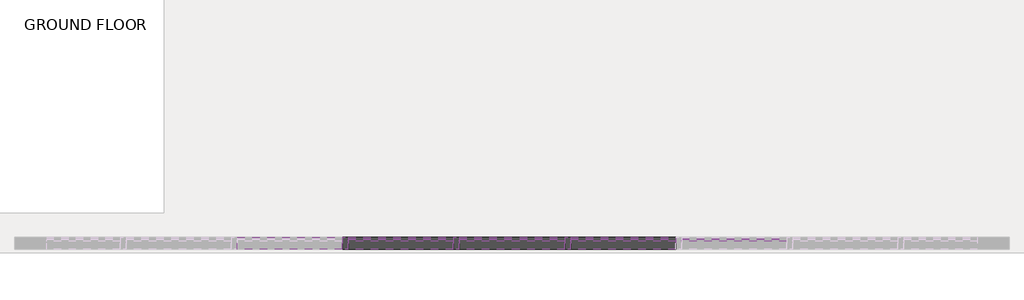
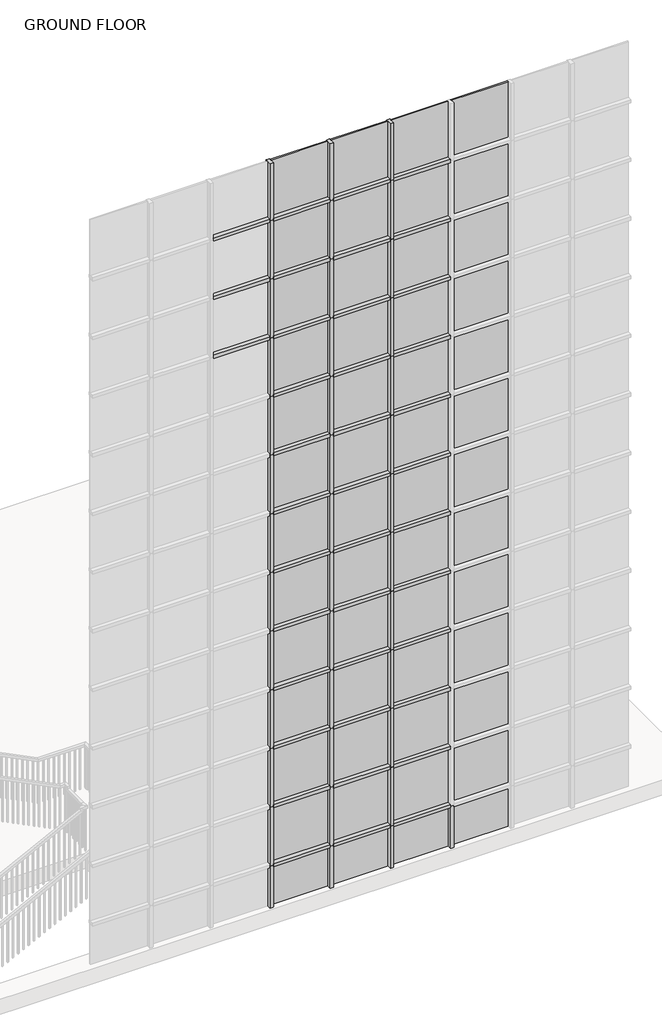
# One storey, part 4 of 16: 79 members, 52 plates.
"""IFC4 building model written with IfcOpenShell, lengths in millimetres."""

from ifc_helpers import new_model, si_unit, origin, place, context, project, spatial, transform, mapped, element, save
from components import member_d518c94e, member_b860638c, member_31fee25f, system_panel_glazed_5cba32e5

model = new_model("IFC4")

# Units and contexts
model_context = context("Model", 3, world=origin())
ifc_project = project(units=[si_unit("LENGTHUNIT", "METRE", prefix="MILLI")], contexts=[model_context])

# Site, building, storey
site = spatial("IfcSite", under=ifc_project)
building = spatial("IfcBuilding", under=site)
storey = spatial("IfcBuildingStorey", under=building, Name="GROUND FLOOR", Elevation=0.0)

# Members
placement = place(None, origin())
member_shape = member_d518c94e(model_context)
element("IfcMember", 1, ObjectType="Rectangular Mullion : 2.5\" x 5\" rectangular", at=placement, inside=storey, context=model_context, shape_type="MappedRepresentation", body=[
    mapped(member_shape, transform((-1030.1171381, -5739.2238032, 1168.8884615), x_axis=(0.0, 0.0, 1.0), y_axis=(0.0, -1.0, 0.0), z_axis=(1.0, 0.0, 0.0))),
])
element("IfcMember", 2, ObjectType="Rectangular Mullion : 2.5\" x 5\" rectangular", at=placement, inside=storey, context=model_context, shape_type="MappedRepresentation", body=[
    mapped(member_shape, transform((135.3520927, -5739.2238032, 1168.8884615), x_axis=(0.0, 0.0, 1.0), y_axis=(0.0, -1.0, 0.0), z_axis=(1.0, 0.0, 0.0))),
])
element("IfcMember", 3, ObjectType="Rectangular Mullion : 2.5\" x 5\" rectangular", at=placement, inside=storey, context=model_context, shape_type="MappedRepresentation", body=[
    mapped(member_shape, transform((1300.8213234, -5739.2238032, 1168.8884615), x_axis=(0.0, 0.0, 1.0), y_axis=(0.0, -1.0, 0.0), z_axis=(1.0, 0.0, 0.0))),
])
element("IfcMember", 4, ObjectType="Rectangular Mullion : 2.5\" x 5\" rectangular", at=placement, inside=storey, context=model_context, shape_type="MappedRepresentation", body=[
    mapped(member_shape, transform((-1030.1171381, -5739.2238032, 2369.5269231), x_axis=(0.0, 0.0, 1.0), y_axis=(0.0, -1.0, 0.0), z_axis=(1.0, 0.0, 0.0))),
])
element("IfcMember", 5, ObjectType="Rectangular Mullion : 2.5\" x 5\" rectangular", at=placement, inside=storey, context=model_context, shape_type="MappedRepresentation", body=[
    mapped(member_shape, transform((135.3520927, -5739.2238032, 2369.5269231), x_axis=(0.0, 0.0, 1.0), y_axis=(0.0, -1.0, 0.0), z_axis=(1.0, 0.0, 0.0))),
])
element("IfcMember", 6, ObjectType="Rectangular Mullion : 2.5\" x 5\" rectangular", at=placement, inside=storey, context=model_context, shape_type="MappedRepresentation", body=[
    mapped(member_shape, transform((1300.8213234, -5739.2238032, 2369.5269231), x_axis=(0.0, 0.0, 1.0), y_axis=(0.0, -1.0, 0.0), z_axis=(1.0, 0.0, 0.0))),
])
element("IfcMember", 7, ObjectType="Rectangular Mullion : 2.5\" x 5\" rectangular", at=placement, inside=storey, context=model_context, shape_type="MappedRepresentation", body=[
    mapped(member_shape, transform((-1030.1171381, -5739.2238032, 3570.1653846), x_axis=(0.0, 0.0, 1.0), y_axis=(0.0, -1.0, 0.0), z_axis=(1.0, 0.0, 0.0))),
])
element("IfcMember", 8, ObjectType="Rectangular Mullion : 2.5\" x 5\" rectangular", at=placement, inside=storey, context=model_context, shape_type="MappedRepresentation", body=[
    mapped(member_shape, transform((135.3520927, -5739.2238032, 3570.1653846), x_axis=(0.0, 0.0, 1.0), y_axis=(0.0, -1.0, 0.0), z_axis=(1.0, 0.0, 0.0))),
])
element("IfcMember", 9, ObjectType="Rectangular Mullion : 2.5\" x 5\" rectangular", at=placement, inside=storey, context=model_context, shape_type="MappedRepresentation", body=[
    mapped(member_shape, transform((1300.8213234, -5739.2238032, 3570.1653846), x_axis=(0.0, 0.0, 1.0), y_axis=(0.0, -1.0, 0.0), z_axis=(1.0, 0.0, 0.0))),
])
element("IfcMember", 10, ObjectType="Rectangular Mullion : 2.5\" x 5\" rectangular", at=placement, inside=storey, context=model_context, shape_type="MappedRepresentation", body=[
    mapped(member_shape, transform((-1030.1171381, -5739.2238032, 4770.8038462), x_axis=(0.0, 0.0, 1.0), y_axis=(0.0, -1.0, 0.0), z_axis=(1.0, 0.0, 0.0))),
])
element("IfcMember", 11, ObjectType="Rectangular Mullion : 2.5\" x 5\" rectangular", at=placement, inside=storey, context=model_context, shape_type="MappedRepresentation", body=[
    mapped(member_shape, transform((135.3520927, -5739.2238032, 4770.8038462), x_axis=(0.0, 0.0, 1.0), y_axis=(0.0, -1.0, 0.0), z_axis=(1.0, 0.0, 0.0))),
])
element("IfcMember", 12, ObjectType="Rectangular Mullion : 2.5\" x 5\" rectangular", at=placement, inside=storey, context=model_context, shape_type="MappedRepresentation", body=[
    mapped(member_shape, transform((1300.8213234, -5739.2238032, 4770.8038462), x_axis=(0.0, 0.0, 1.0), y_axis=(0.0, -1.0, 0.0), z_axis=(1.0, 0.0, 0.0))),
])
element("IfcMember", 13, ObjectType="Rectangular Mullion : 2.5\" x 5\" rectangular", at=placement, inside=storey, context=model_context, shape_type="MappedRepresentation", body=[
    mapped(member_shape, transform((-1030.1171381, -5739.2238032, 5971.4423077), x_axis=(0.0, 0.0, 1.0), y_axis=(0.0, -1.0, 0.0), z_axis=(1.0, 0.0, 0.0))),
])
element("IfcMember", 14, ObjectType="Rectangular Mullion : 2.5\" x 5\" rectangular", at=placement, inside=storey, context=model_context, shape_type="MappedRepresentation", body=[
    mapped(member_shape, transform((135.3520927, -5739.2238032, 5971.4423077), x_axis=(0.0, 0.0, 1.0), y_axis=(0.0, -1.0, 0.0), z_axis=(1.0, 0.0, 0.0))),
])
element("IfcMember", 15, ObjectType="Rectangular Mullion : 2.5\" x 5\" rectangular", at=placement, inside=storey, context=model_context, shape_type="MappedRepresentation", body=[
    mapped(member_shape, transform((1300.8213234, -5739.2238032, 5971.4423077), x_axis=(0.0, 0.0, 1.0), y_axis=(0.0, -1.0, 0.0), z_axis=(1.0, 0.0, 0.0))),
])
element("IfcMember", 16, ObjectType="Rectangular Mullion : 2.5\" x 5\" rectangular", at=placement, inside=storey, context=model_context, shape_type="MappedRepresentation", body=[
    mapped(member_shape, transform((-1030.1171381, -5739.2238032, 7172.0807692), x_axis=(0.0, 0.0, 1.0), y_axis=(0.0, -1.0, 0.0), z_axis=(1.0, 0.0, 0.0))),
])
element("IfcMember", 17, ObjectType="Rectangular Mullion : 2.5\" x 5\" rectangular", at=placement, inside=storey, context=model_context, shape_type="MappedRepresentation", body=[
    mapped(member_shape, transform((135.3520927, -5739.2238032, 7172.0807692), x_axis=(0.0, 0.0, 1.0), y_axis=(0.0, -1.0, 0.0), z_axis=(1.0, 0.0, 0.0))),
])
element("IfcMember", 18, ObjectType="Rectangular Mullion : 2.5\" x 5\" rectangular", at=placement, inside=storey, context=model_context, shape_type="MappedRepresentation", body=[
    mapped(member_shape, transform((1300.8213234, -5739.2238032, 7172.0807692), x_axis=(0.0, 0.0, 1.0), y_axis=(0.0, -1.0, 0.0), z_axis=(1.0, 0.0, 0.0))),
])
element("IfcMember", 19, ObjectType="Rectangular Mullion : 2.5\" x 5\" rectangular", at=placement, inside=storey, context=model_context, shape_type="MappedRepresentation", body=[
    mapped(member_shape, transform((-1030.1171381, -5739.2238032, 8372.7192308), x_axis=(0.0, 0.0, 1.0), y_axis=(0.0, -1.0, 0.0), z_axis=(1.0, 0.0, 0.0))),
])
element("IfcMember", 20, ObjectType="Rectangular Mullion : 2.5\" x 5\" rectangular", at=placement, inside=storey, context=model_context, shape_type="MappedRepresentation", body=[
    mapped(member_shape, transform((135.3520927, -5739.2238032, 8372.7192308), x_axis=(0.0, 0.0, 1.0), y_axis=(0.0, -1.0, 0.0), z_axis=(1.0, 0.0, 0.0))),
])
element("IfcMember", 21, ObjectType="Rectangular Mullion : 2.5\" x 5\" rectangular", at=placement, inside=storey, context=model_context, shape_type="MappedRepresentation", body=[
    mapped(member_shape, transform((1300.8213234, -5739.2238032, 8372.7192308), x_axis=(0.0, 0.0, 1.0), y_axis=(0.0, -1.0, 0.0), z_axis=(1.0, 0.0, 0.0))),
])
element("IfcMember", 22, ObjectType="Rectangular Mullion : 2.5\" x 5\" rectangular", at=placement, inside=storey, context=model_context, shape_type="MappedRepresentation", body=[
    mapped(member_shape, transform((-1030.1171381, -5739.2238032, 9573.3576923), x_axis=(0.0, 0.0, 1.0), y_axis=(0.0, -1.0, 0.0), z_axis=(1.0, 0.0, 0.0))),
])
element("IfcMember", 23, ObjectType="Rectangular Mullion : 2.5\" x 5\" rectangular", at=placement, inside=storey, context=model_context, shape_type="MappedRepresentation", body=[
    mapped(member_shape, transform((135.3520927, -5739.2238032, 9573.3576923), x_axis=(0.0, 0.0, 1.0), y_axis=(0.0, -1.0, 0.0), z_axis=(1.0, 0.0, 0.0))),
])
element("IfcMember", 24, ObjectType="Rectangular Mullion : 2.5\" x 5\" rectangular", at=placement, inside=storey, context=model_context, shape_type="MappedRepresentation", body=[
    mapped(member_shape, transform((1300.8213234, -5739.2238032, 9573.3576923), x_axis=(0.0, 0.0, 1.0), y_axis=(0.0, -1.0, 0.0), z_axis=(1.0, 0.0, 0.0))),
])
element("IfcMember", 25, ObjectType="Rectangular Mullion : 2.5\" x 5\" rectangular", at=placement, inside=storey, context=model_context, shape_type="MappedRepresentation", body=[
    mapped(member_shape, transform((-1030.1171381, -5739.2238032, 10773.9961538), x_axis=(0.0, 0.0, 1.0), y_axis=(0.0, -1.0, 0.0), z_axis=(1.0, 0.0, 0.0))),
])
element("IfcMember", 26, ObjectType="Rectangular Mullion : 2.5\" x 5\" rectangular", at=placement, inside=storey, context=model_context, shape_type="MappedRepresentation", body=[
    mapped(member_shape, transform((135.3520927, -5739.2238032, 10773.9961538), x_axis=(0.0, 0.0, 1.0), y_axis=(0.0, -1.0, 0.0), z_axis=(1.0, 0.0, 0.0))),
])
element("IfcMember", 27, ObjectType="Rectangular Mullion : 2.5\" x 5\" rectangular", at=placement, inside=storey, context=model_context, shape_type="MappedRepresentation", body=[
    mapped(member_shape, transform((1300.8213234, -5739.2238032, 10773.9961538), x_axis=(0.0, 0.0, 1.0), y_axis=(0.0, -1.0, 0.0), z_axis=(1.0, 0.0, 0.0))),
])
element("IfcMember", 28, ObjectType="Rectangular Mullion : 2.5\" x 5\" rectangular", at=placement, inside=storey, context=model_context, shape_type="MappedRepresentation", body=[
    mapped(member_shape, transform((-2195.5863688, -5739.2238032, 11974.6346154), x_axis=(0.0, 0.0, 1.0), y_axis=(0.0, -1.0, 0.0), z_axis=(1.0, 0.0, 0.0))),
])
element("IfcMember", 29, ObjectType="Rectangular Mullion : 2.5\" x 5\" rectangular", at=placement, inside=storey, context=model_context, shape_type="MappedRepresentation", body=[
    mapped(member_shape, transform((-1030.1171381, -5739.2238032, 11974.6346154), x_axis=(0.0, 0.0, 1.0), y_axis=(0.0, -1.0, 0.0), z_axis=(1.0, 0.0, 0.0))),
])
element("IfcMember", 30, ObjectType="Rectangular Mullion : 2.5\" x 5\" rectangular", at=placement, inside=storey, context=model_context, shape_type="MappedRepresentation", body=[
    mapped(member_shape, transform((135.3520927, -5739.2238032, 11974.6346154), x_axis=(0.0, 0.0, 1.0), y_axis=(0.0, -1.0, 0.0), z_axis=(1.0, 0.0, 0.0))),
])
element("IfcMember", 31, ObjectType="Rectangular Mullion : 2.5\" x 5\" rectangular", at=placement, inside=storey, context=model_context, shape_type="MappedRepresentation", body=[
    mapped(member_shape, transform((1300.8213234, -5739.2238032, 11974.6346154), x_axis=(0.0, 0.0, 1.0), y_axis=(0.0, -1.0, 0.0), z_axis=(1.0, 0.0, 0.0))),
])
element("IfcMember", 32, ObjectType="Rectangular Mullion : 2.5\" x 5\" rectangular", at=placement, inside=storey, context=model_context, shape_type="MappedRepresentation", body=[
    mapped(member_shape, transform((-2195.5863688, -5739.2238032, 13175.2730769), x_axis=(0.0, 0.0, 1.0), y_axis=(0.0, -1.0, 0.0), z_axis=(1.0, 0.0, 0.0))),
])
element("IfcMember", 33, ObjectType="Rectangular Mullion : 2.5\" x 5\" rectangular", at=placement, inside=storey, context=model_context, shape_type="MappedRepresentation", body=[
    mapped(member_shape, transform((-1030.1171381, -5739.2238032, 13175.2730769), x_axis=(0.0, 0.0, 1.0), y_axis=(0.0, -1.0, 0.0), z_axis=(1.0, 0.0, 0.0))),
])
element("IfcMember", 34, ObjectType="Rectangular Mullion : 2.5\" x 5\" rectangular", at=placement, inside=storey, context=model_context, shape_type="MappedRepresentation", body=[
    mapped(member_shape, transform((135.3520927, -5739.2238032, 13175.2730769), x_axis=(0.0, 0.0, 1.0), y_axis=(0.0, -1.0, 0.0), z_axis=(1.0, 0.0, 0.0))),
])
element("IfcMember", 35, ObjectType="Rectangular Mullion : 2.5\" x 5\" rectangular", at=placement, inside=storey, context=model_context, shape_type="MappedRepresentation", body=[
    mapped(member_shape, transform((1300.8213234, -5739.2238032, 13175.2730769), x_axis=(0.0, 0.0, 1.0), y_axis=(0.0, -1.0, 0.0), z_axis=(1.0, 0.0, 0.0))),
])
element("IfcMember", 36, ObjectType="Rectangular Mullion : 2.5\" x 5\" rectangular", at=placement, inside=storey, context=model_context, shape_type="MappedRepresentation", body=[
    mapped(member_shape, transform((-2195.5863688, -5739.2238032, 14375.9115385), x_axis=(0.0, 0.0, 1.0), y_axis=(0.0, -1.0, 0.0), z_axis=(1.0, 0.0, 0.0))),
])
element("IfcMember", 37, ObjectType="Rectangular Mullion : 2.5\" x 5\" rectangular", at=placement, inside=storey, context=model_context, shape_type="MappedRepresentation", body=[
    mapped(member_shape, transform((-1030.1171381, -5739.2238032, 14375.9115385), x_axis=(0.0, 0.0, 1.0), y_axis=(0.0, -1.0, 0.0), z_axis=(1.0, 0.0, 0.0))),
])
element("IfcMember", 38, ObjectType="Rectangular Mullion : 2.5\" x 5\" rectangular", at=placement, inside=storey, context=model_context, shape_type="MappedRepresentation", body=[
    mapped(member_shape, transform((135.3520927, -5739.2238032, 14375.9115385), x_axis=(0.0, 0.0, 1.0), y_axis=(0.0, -1.0, 0.0), z_axis=(1.0, 0.0, 0.0))),
])
element("IfcMember", 39, ObjectType="Rectangular Mullion : 2.5\" x 5\" rectangular", at=placement, inside=storey, context=model_context, shape_type="MappedRepresentation", body=[
    mapped(member_shape, transform((1300.8213234, -5739.2238032, 14375.9115385), x_axis=(0.0, 0.0, 1.0), y_axis=(0.0, -1.0, 0.0), z_axis=(1.0, 0.0, 0.0))),
])
member_2_shape = member_b860638c(model_context)
element("IfcMember", 40, ObjectType="Rectangular Mullion : 2.5\" x 5\" rectangular", at=placement, inside=storey, context=model_context, shape_type="MappedRepresentation", body=[
    mapped(member_2_shape, transform((-2163.8363688, -5739.2238032, 0.0), x_axis=(1.0, 0.0, 0.0), y_axis=(0.0, -1.0, 0.0), z_axis=(0.0, 0.0, -1.0))),
])
element("IfcMember", 41, ObjectType="Rectangular Mullion : 2.5\" x 5\" rectangular", at=placement, inside=storey, context=model_context, shape_type="MappedRepresentation", body=[
    mapped(member_2_shape, transform((-998.3671381, -5739.2238032, 0.0), x_axis=(1.0, 0.0, 0.0), y_axis=(0.0, -1.0, 0.0), z_axis=(0.0, 0.0, -1.0))),
])
element("IfcMember", 42, ObjectType="Rectangular Mullion : 2.5\" x 5\" rectangular", at=placement, inside=storey, context=model_context, shape_type="MappedRepresentation", body=[
    mapped(member_2_shape, transform((167.1020927, -5739.2238032, 0.0), x_axis=(1.0, 0.0, 0.0), y_axis=(0.0, -1.0, 0.0), z_axis=(0.0, 0.0, -1.0))),
])
element("IfcMember", 43, ObjectType="Rectangular Mullion : 2.5\" x 5\" rectangular", at=placement, inside=storey, context=model_context, shape_type="MappedRepresentation", body=[
    mapped(member_2_shape, transform((1332.5713234, -5739.2238032, 0.0), x_axis=(1.0, 0.0, 0.0), y_axis=(0.0, -1.0, 0.0), z_axis=(0.0, 0.0, -1.0))),
])
member_3_shape = member_31fee25f(model_context)
element("IfcMember", 44, ObjectType="Rectangular Mullion : 2.5\" x 5\" rectangular", at=placement, inside=storey, context=model_context, shape_type="MappedRepresentation", body=[
    mapped(member_3_shape, transform((-2163.8363688, -5739.2238032, 1168.8884615), x_axis=(1.0, 0.0, 0.0), y_axis=(0.0, -1.0, 0.0), z_axis=(0.0, 0.0, -1.0))),
])
element("IfcMember", 45, ObjectType="Rectangular Mullion : 2.5\" x 5\" rectangular", at=placement, inside=storey, context=model_context, shape_type="MappedRepresentation", body=[
    mapped(member_3_shape, transform((-998.3671381, -5739.2238032, 1168.8884615), x_axis=(1.0, 0.0, 0.0), y_axis=(0.0, -1.0, 0.0), z_axis=(0.0, 0.0, -1.0))),
])
element("IfcMember", 46, ObjectType="Rectangular Mullion : 2.5\" x 5\" rectangular", at=placement, inside=storey, context=model_context, shape_type="MappedRepresentation", body=[
    mapped(member_3_shape, transform((167.1020927, -5739.2238032, 1168.8884615), x_axis=(1.0, 0.0, 0.0), y_axis=(0.0, -1.0, 0.0), z_axis=(0.0, 0.0, -1.0))),
])
element("IfcMember", 47, ObjectType="Rectangular Mullion : 2.5\" x 5\" rectangular", at=placement, inside=storey, context=model_context, shape_type="MappedRepresentation", body=[
    mapped(member_3_shape, transform((-2163.8363688, -5739.2238032, 2369.5269231), x_axis=(1.0, 0.0, 0.0), y_axis=(0.0, -1.0, 0.0), z_axis=(0.0, 0.0, -1.0))),
])
element("IfcMember", 48, ObjectType="Rectangular Mullion : 2.5\" x 5\" rectangular", at=placement, inside=storey, context=model_context, shape_type="MappedRepresentation", body=[
    mapped(member_3_shape, transform((-998.3671381, -5739.2238032, 2369.5269231), x_axis=(1.0, 0.0, 0.0), y_axis=(0.0, -1.0, 0.0), z_axis=(0.0, 0.0, -1.0))),
])
element("IfcMember", 49, ObjectType="Rectangular Mullion : 2.5\" x 5\" rectangular", at=placement, inside=storey, context=model_context, shape_type="MappedRepresentation", body=[
    mapped(member_3_shape, transform((167.1020927, -5739.2238032, 2369.5269231), x_axis=(1.0, 0.0, 0.0), y_axis=(0.0, -1.0, 0.0), z_axis=(0.0, 0.0, -1.0))),
])
element("IfcMember", 50, ObjectType="Rectangular Mullion : 2.5\" x 5\" rectangular", at=placement, inside=storey, context=model_context, shape_type="MappedRepresentation", body=[
    mapped(member_3_shape, transform((-2163.8363688, -5739.2238032, 3570.1653846), x_axis=(1.0, 0.0, 0.0), y_axis=(0.0, -1.0, 0.0), z_axis=(0.0, 0.0, -1.0))),
])
element("IfcMember", 51, ObjectType="Rectangular Mullion : 2.5\" x 5\" rectangular", at=placement, inside=storey, context=model_context, shape_type="MappedRepresentation", body=[
    mapped(member_3_shape, transform((-998.3671381, -5739.2238032, 3570.1653846), x_axis=(1.0, 0.0, 0.0), y_axis=(0.0, -1.0, 0.0), z_axis=(0.0, 0.0, -1.0))),
])
element("IfcMember", 52, ObjectType="Rectangular Mullion : 2.5\" x 5\" rectangular", at=placement, inside=storey, context=model_context, shape_type="MappedRepresentation", body=[
    mapped(member_3_shape, transform((167.1020927, -5739.2238032, 3570.1653846), x_axis=(1.0, 0.0, 0.0), y_axis=(0.0, -1.0, 0.0), z_axis=(0.0, 0.0, -1.0))),
])
element("IfcMember", 53, ObjectType="Rectangular Mullion : 2.5\" x 5\" rectangular", at=placement, inside=storey, context=model_context, shape_type="MappedRepresentation", body=[
    mapped(member_3_shape, transform((-2163.8363688, -5739.2238032, 4770.8038462), x_axis=(1.0, 0.0, 0.0), y_axis=(0.0, -1.0, 0.0), z_axis=(0.0, 0.0, -1.0))),
])
element("IfcMember", 54, ObjectType="Rectangular Mullion : 2.5\" x 5\" rectangular", at=placement, inside=storey, context=model_context, shape_type="MappedRepresentation", body=[
    mapped(member_3_shape, transform((-998.3671381, -5739.2238032, 4770.8038462), x_axis=(1.0, 0.0, 0.0), y_axis=(0.0, -1.0, 0.0), z_axis=(0.0, 0.0, -1.0))),
])
element("IfcMember", 55, ObjectType="Rectangular Mullion : 2.5\" x 5\" rectangular", at=placement, inside=storey, context=model_context, shape_type="MappedRepresentation", body=[
    mapped(member_3_shape, transform((167.1020927, -5739.2238032, 4770.8038462), x_axis=(1.0, 0.0, 0.0), y_axis=(0.0, -1.0, 0.0), z_axis=(0.0, 0.0, -1.0))),
])
element("IfcMember", 56, ObjectType="Rectangular Mullion : 2.5\" x 5\" rectangular", at=placement, inside=storey, context=model_context, shape_type="MappedRepresentation", body=[
    mapped(member_3_shape, transform((-2163.8363688, -5739.2238032, 5971.4423077), x_axis=(1.0, 0.0, 0.0), y_axis=(0.0, -1.0, 0.0), z_axis=(0.0, 0.0, -1.0))),
])
element("IfcMember", 57, ObjectType="Rectangular Mullion : 2.5\" x 5\" rectangular", at=placement, inside=storey, context=model_context, shape_type="MappedRepresentation", body=[
    mapped(member_3_shape, transform((-998.3671381, -5739.2238032, 5971.4423077), x_axis=(1.0, 0.0, 0.0), y_axis=(0.0, -1.0, 0.0), z_axis=(0.0, 0.0, -1.0))),
])
element("IfcMember", 58, ObjectType="Rectangular Mullion : 2.5\" x 5\" rectangular", at=placement, inside=storey, context=model_context, shape_type="MappedRepresentation", body=[
    mapped(member_3_shape, transform((167.1020927, -5739.2238032, 5971.4423077), x_axis=(1.0, 0.0, 0.0), y_axis=(0.0, -1.0, 0.0), z_axis=(0.0, 0.0, -1.0))),
])
element("IfcMember", 59, ObjectType="Rectangular Mullion : 2.5\" x 5\" rectangular", at=placement, inside=storey, context=model_context, shape_type="MappedRepresentation", body=[
    mapped(member_3_shape, transform((-2163.8363688, -5739.2238032, 7172.0807692), x_axis=(1.0, 0.0, 0.0), y_axis=(0.0, -1.0, 0.0), z_axis=(0.0, 0.0, -1.0))),
])
element("IfcMember", 60, ObjectType="Rectangular Mullion : 2.5\" x 5\" rectangular", at=placement, inside=storey, context=model_context, shape_type="MappedRepresentation", body=[
    mapped(member_3_shape, transform((-998.3671381, -5739.2238032, 7172.0807692), x_axis=(1.0, 0.0, 0.0), y_axis=(0.0, -1.0, 0.0), z_axis=(0.0, 0.0, -1.0))),
])
element("IfcMember", 61, ObjectType="Rectangular Mullion : 2.5\" x 5\" rectangular", at=placement, inside=storey, context=model_context, shape_type="MappedRepresentation", body=[
    mapped(member_3_shape, transform((167.1020927, -5739.2238032, 7172.0807692), x_axis=(1.0, 0.0, 0.0), y_axis=(0.0, -1.0, 0.0), z_axis=(0.0, 0.0, -1.0))),
])
element("IfcMember", 62, ObjectType="Rectangular Mullion : 2.5\" x 5\" rectangular", at=placement, inside=storey, context=model_context, shape_type="MappedRepresentation", body=[
    mapped(member_3_shape, transform((-2163.8363688, -5739.2238032, 8372.7192308), x_axis=(1.0, 0.0, 0.0), y_axis=(0.0, -1.0, 0.0), z_axis=(0.0, 0.0, -1.0))),
])
element("IfcMember", 63, ObjectType="Rectangular Mullion : 2.5\" x 5\" rectangular", at=placement, inside=storey, context=model_context, shape_type="MappedRepresentation", body=[
    mapped(member_3_shape, transform((-998.3671381, -5739.2238032, 8372.7192308), x_axis=(1.0, 0.0, 0.0), y_axis=(0.0, -1.0, 0.0), z_axis=(0.0, 0.0, -1.0))),
])
element("IfcMember", 64, ObjectType="Rectangular Mullion : 2.5\" x 5\" rectangular", at=placement, inside=storey, context=model_context, shape_type="MappedRepresentation", body=[
    mapped(member_3_shape, transform((167.1020927, -5739.2238032, 8372.7192308), x_axis=(1.0, 0.0, 0.0), y_axis=(0.0, -1.0, 0.0), z_axis=(0.0, 0.0, -1.0))),
])
element("IfcMember", 65, ObjectType="Rectangular Mullion : 2.5\" x 5\" rectangular", at=placement, inside=storey, context=model_context, shape_type="MappedRepresentation", body=[
    mapped(member_3_shape, transform((-2163.8363688, -5739.2238032, 9573.3576923), x_axis=(1.0, 0.0, 0.0), y_axis=(0.0, -1.0, 0.0), z_axis=(0.0, 0.0, -1.0))),
])
element("IfcMember", 66, ObjectType="Rectangular Mullion : 2.5\" x 5\" rectangular", at=placement, inside=storey, context=model_context, shape_type="MappedRepresentation", body=[
    mapped(member_3_shape, transform((-998.3671381, -5739.2238032, 9573.3576923), x_axis=(1.0, 0.0, 0.0), y_axis=(0.0, -1.0, 0.0), z_axis=(0.0, 0.0, -1.0))),
])
element("IfcMember", 67, ObjectType="Rectangular Mullion : 2.5\" x 5\" rectangular", at=placement, inside=storey, context=model_context, shape_type="MappedRepresentation", body=[
    mapped(member_3_shape, transform((167.1020927, -5739.2238032, 9573.3576923), x_axis=(1.0, 0.0, 0.0), y_axis=(0.0, -1.0, 0.0), z_axis=(0.0, 0.0, -1.0))),
])
element("IfcMember", 68, ObjectType="Rectangular Mullion : 2.5\" x 5\" rectangular", at=placement, inside=storey, context=model_context, shape_type="MappedRepresentation", body=[
    mapped(member_3_shape, transform((-2163.8363688, -5739.2238032, 10773.9961538), x_axis=(1.0, 0.0, 0.0), y_axis=(0.0, -1.0, 0.0), z_axis=(0.0, 0.0, -1.0))),
])
element("IfcMember", 69, ObjectType="Rectangular Mullion : 2.5\" x 5\" rectangular", at=placement, inside=storey, context=model_context, shape_type="MappedRepresentation", body=[
    mapped(member_3_shape, transform((-998.3671381, -5739.2238032, 10773.9961538), x_axis=(1.0, 0.0, 0.0), y_axis=(0.0, -1.0, 0.0), z_axis=(0.0, 0.0, -1.0))),
])
element("IfcMember", 70, ObjectType="Rectangular Mullion : 2.5\" x 5\" rectangular", at=placement, inside=storey, context=model_context, shape_type="MappedRepresentation", body=[
    mapped(member_3_shape, transform((167.1020927, -5739.2238032, 10773.9961538), x_axis=(1.0, 0.0, 0.0), y_axis=(0.0, -1.0, 0.0), z_axis=(0.0, 0.0, -1.0))),
])
element("IfcMember", 71, ObjectType="Rectangular Mullion : 2.5\" x 5\" rectangular", at=placement, inside=storey, context=model_context, shape_type="MappedRepresentation", body=[
    mapped(member_3_shape, transform((-2163.8363688, -5739.2238032, 11974.6346154), x_axis=(1.0, 0.0, 0.0), y_axis=(0.0, -1.0, 0.0), z_axis=(0.0, 0.0, -1.0))),
])
element("IfcMember", 72, ObjectType="Rectangular Mullion : 2.5\" x 5\" rectangular", at=placement, inside=storey, context=model_context, shape_type="MappedRepresentation", body=[
    mapped(member_3_shape, transform((-998.3671381, -5739.2238032, 11974.6346154), x_axis=(1.0, 0.0, 0.0), y_axis=(0.0, -1.0, 0.0), z_axis=(0.0, 0.0, -1.0))),
])
element("IfcMember", 73, ObjectType="Rectangular Mullion : 2.5\" x 5\" rectangular", at=placement, inside=storey, context=model_context, shape_type="MappedRepresentation", body=[
    mapped(member_3_shape, transform((167.1020927, -5739.2238032, 11974.6346154), x_axis=(1.0, 0.0, 0.0), y_axis=(0.0, -1.0, 0.0), z_axis=(0.0, 0.0, -1.0))),
])
element("IfcMember", 74, ObjectType="Rectangular Mullion : 2.5\" x 5\" rectangular", at=placement, inside=storey, context=model_context, shape_type="MappedRepresentation", body=[
    mapped(member_3_shape, transform((-2163.8363688, -5739.2238032, 13175.2730769), x_axis=(1.0, 0.0, 0.0), y_axis=(0.0, -1.0, 0.0), z_axis=(0.0, 0.0, -1.0))),
])
element("IfcMember", 75, ObjectType="Rectangular Mullion : 2.5\" x 5\" rectangular", at=placement, inside=storey, context=model_context, shape_type="MappedRepresentation", body=[
    mapped(member_3_shape, transform((-998.3671381, -5739.2238032, 13175.2730769), x_axis=(1.0, 0.0, 0.0), y_axis=(0.0, -1.0, 0.0), z_axis=(0.0, 0.0, -1.0))),
])
element("IfcMember", 76, ObjectType="Rectangular Mullion : 2.5\" x 5\" rectangular", at=placement, inside=storey, context=model_context, shape_type="MappedRepresentation", body=[
    mapped(member_3_shape, transform((167.1020927, -5739.2238032, 13175.2730769), x_axis=(1.0, 0.0, 0.0), y_axis=(0.0, -1.0, 0.0), z_axis=(0.0, 0.0, -1.0))),
])
element("IfcMember", 77, ObjectType="Rectangular Mullion : 2.5\" x 5\" rectangular", at=placement, inside=storey, context=model_context, shape_type="MappedRepresentation", body=[
    mapped(member_2_shape, transform((-2163.8363688, -5739.2238032, 14375.9115385), x_axis=(1.0, 0.0, 0.0), y_axis=(0.0, -1.0, 0.0), z_axis=(0.0, 0.0, -1.0))),
])
element("IfcMember", 78, ObjectType="Rectangular Mullion : 2.5\" x 5\" rectangular", at=placement, inside=storey, context=model_context, shape_type="MappedRepresentation", body=[
    mapped(member_2_shape, transform((-998.3671381, -5739.2238032, 14375.9115385), x_axis=(1.0, 0.0, 0.0), y_axis=(0.0, -1.0, 0.0), z_axis=(0.0, 0.0, -1.0))),
])
element("IfcMember", 79, ObjectType="Rectangular Mullion : 2.5\" x 5\" rectangular", at=placement, inside=storey, context=model_context, shape_type="MappedRepresentation", body=[
    mapped(member_2_shape, transform((167.1020927, -5739.2238032, 14375.9115385), x_axis=(1.0, 0.0, 0.0), y_axis=(0.0, -1.0, 0.0), z_axis=(0.0, 0.0, -1.0))),
])

# Plates
system_panel_glazed_shape = system_panel_glazed_5cba32e5(model_context)
element("IfcPlate", 80, ObjectType="System Panel : Glazed", at=placement, inside=storey, context=model_context, shape_type="MappedRepresentation", body=[
    mapped(system_panel_glazed_shape, transform((-1581.1017534, -5739.2238032, 0.0), x_axis=(1.0, 0.0, 0.0), y_axis=(0.0, 1.0, 0.0), z_axis=(0.0, 0.0, 1.0))),
])
element("IfcPlate", 81, ObjectType="System Panel : Glazed", at=placement, inside=storey, context=model_context, shape_type="MappedRepresentation", body=[
    mapped(system_panel_glazed_shape, transform((-415.6325227, -5739.2238032, 0.0), x_axis=(1.0, 0.0, 0.0), y_axis=(0.0, 1.0, 0.0), z_axis=(0.0, 0.0, 1.0))),
])
element("IfcPlate", 82, ObjectType="System Panel : Glazed", at=placement, inside=storey, context=model_context, shape_type="MappedRepresentation", body=[
    mapped(system_panel_glazed_shape, transform((749.836708, -5739.2238032, 0.0), x_axis=(1.0, 0.0, 0.0), y_axis=(0.0, 1.0, 0.0), z_axis=(0.0, 0.0, 1.0))),
])
element("IfcPlate", 83, ObjectType="System Panel : Glazed", at=placement, inside=storey, context=model_context, shape_type="MappedRepresentation", body=[
    mapped(system_panel_glazed_shape, transform((1915.3059387, -5739.2238032, 0.0), x_axis=(1.0, 0.0, 0.0), y_axis=(0.0, 1.0, 0.0), z_axis=(0.0, 0.0, 1.0))),
])
element("IfcPlate", 84, ObjectType="System Panel : Glazed", at=placement, inside=storey, context=model_context, shape_type="MappedRepresentation", body=[
    mapped(system_panel_glazed_shape, transform((-1581.1017534, -5739.2238032, 1200.6384615), x_axis=(1.0, 0.0, 0.0), y_axis=(0.0, 1.0, 0.0), z_axis=(0.0, 0.0, 1.0))),
])
element("IfcPlate", 85, ObjectType="System Panel : Glazed", at=placement, inside=storey, context=model_context, shape_type="MappedRepresentation", body=[
    mapped(system_panel_glazed_shape, transform((-415.6325227, -5739.2238032, 1200.6384615), x_axis=(1.0, 0.0, 0.0), y_axis=(0.0, 1.0, 0.0), z_axis=(0.0, 0.0, 1.0))),
])
element("IfcPlate", 86, ObjectType="System Panel : Glazed", at=placement, inside=storey, context=model_context, shape_type="MappedRepresentation", body=[
    mapped(system_panel_glazed_shape, transform((749.836708, -5739.2238032, 1200.6384615), x_axis=(1.0, 0.0, 0.0), y_axis=(0.0, 1.0, 0.0), z_axis=(0.0, 0.0, 1.0))),
])
element("IfcPlate", 87, ObjectType="System Panel : Glazed", at=placement, inside=storey, context=model_context, shape_type="MappedRepresentation", body=[
    mapped(system_panel_glazed_shape, transform((1915.3059387, -5739.2238032, 1200.6384615), x_axis=(1.0, 0.0, 0.0), y_axis=(0.0, 1.0, 0.0), z_axis=(0.0, 0.0, 1.0))),
])
element("IfcPlate", 88, ObjectType="System Panel : Glazed", at=placement, inside=storey, context=model_context, shape_type="MappedRepresentation", body=[
    mapped(system_panel_glazed_shape, transform((-1581.1017534, -5739.2238032, 2401.2769231), x_axis=(1.0, 0.0, 0.0), y_axis=(0.0, 1.0, 0.0), z_axis=(0.0, 0.0, 1.0))),
])
element("IfcPlate", 89, ObjectType="System Panel : Glazed", at=placement, inside=storey, context=model_context, shape_type="MappedRepresentation", body=[
    mapped(system_panel_glazed_shape, transform((-415.6325227, -5739.2238032, 2401.2769231), x_axis=(1.0, 0.0, 0.0), y_axis=(0.0, 1.0, 0.0), z_axis=(0.0, 0.0, 1.0))),
])
element("IfcPlate", 90, ObjectType="System Panel : Glazed", at=placement, inside=storey, context=model_context, shape_type="MappedRepresentation", body=[
    mapped(system_panel_glazed_shape, transform((749.836708, -5739.2238032, 2401.2769231), x_axis=(1.0, 0.0, 0.0), y_axis=(0.0, 1.0, 0.0), z_axis=(0.0, 0.0, 1.0))),
])
element("IfcPlate", 91, ObjectType="System Panel : Glazed", at=placement, inside=storey, context=model_context, shape_type="MappedRepresentation", body=[
    mapped(system_panel_glazed_shape, transform((1915.3059387, -5739.2238032, 2401.2769231), x_axis=(1.0, 0.0, 0.0), y_axis=(0.0, 1.0, 0.0), z_axis=(0.0, 0.0, 1.0))),
])
element("IfcPlate", 92, ObjectType="System Panel : Glazed", at=placement, inside=storey, context=model_context, shape_type="MappedRepresentation", body=[
    mapped(system_panel_glazed_shape, transform((-1581.1017534, -5739.2238032, 3601.9153846), x_axis=(1.0, 0.0, 0.0), y_axis=(0.0, 1.0, 0.0), z_axis=(0.0, 0.0, 1.0))),
])
element("IfcPlate", 93, ObjectType="System Panel : Glazed", at=placement, inside=storey, context=model_context, shape_type="MappedRepresentation", body=[
    mapped(system_panel_glazed_shape, transform((-415.6325227, -5739.2238032, 3601.9153846), x_axis=(1.0, 0.0, 0.0), y_axis=(0.0, 1.0, 0.0), z_axis=(0.0, 0.0, 1.0))),
])
element("IfcPlate", 94, ObjectType="System Panel : Glazed", at=placement, inside=storey, context=model_context, shape_type="MappedRepresentation", body=[
    mapped(system_panel_glazed_shape, transform((749.836708, -5739.2238032, 3601.9153846), x_axis=(1.0, 0.0, 0.0), y_axis=(0.0, 1.0, 0.0), z_axis=(0.0, 0.0, 1.0))),
])
element("IfcPlate", 95, ObjectType="System Panel : Glazed", at=placement, inside=storey, context=model_context, shape_type="MappedRepresentation", body=[
    mapped(system_panel_glazed_shape, transform((1915.3059387, -5739.2238032, 3601.9153846), x_axis=(1.0, 0.0, 0.0), y_axis=(0.0, 1.0, 0.0), z_axis=(0.0, 0.0, 1.0))),
])
element("IfcPlate", 96, ObjectType="System Panel : Glazed", at=placement, inside=storey, context=model_context, shape_type="MappedRepresentation", body=[
    mapped(system_panel_glazed_shape, transform((-1581.1017534, -5739.2238032, 4802.5538462), x_axis=(1.0, 0.0, 0.0), y_axis=(0.0, 1.0, 0.0), z_axis=(0.0, 0.0, 1.0))),
])
element("IfcPlate", 97, ObjectType="System Panel : Glazed", at=placement, inside=storey, context=model_context, shape_type="MappedRepresentation", body=[
    mapped(system_panel_glazed_shape, transform((-415.6325227, -5739.2238032, 4802.5538462), x_axis=(1.0, 0.0, 0.0), y_axis=(0.0, 1.0, 0.0), z_axis=(0.0, 0.0, 1.0))),
])
element("IfcPlate", 98, ObjectType="System Panel : Glazed", at=placement, inside=storey, context=model_context, shape_type="MappedRepresentation", body=[
    mapped(system_panel_glazed_shape, transform((749.836708, -5739.2238032, 4802.5538462), x_axis=(1.0, 0.0, 0.0), y_axis=(0.0, 1.0, 0.0), z_axis=(0.0, 0.0, 1.0))),
])
element("IfcPlate", 99, ObjectType="System Panel : Glazed", at=placement, inside=storey, context=model_context, shape_type="MappedRepresentation", body=[
    mapped(system_panel_glazed_shape, transform((1915.3059387, -5739.2238032, 4802.5538462), x_axis=(1.0, 0.0, 0.0), y_axis=(0.0, 1.0, 0.0), z_axis=(0.0, 0.0, 1.0))),
])
element("IfcPlate", 100, ObjectType="System Panel : Glazed", at=placement, inside=storey, context=model_context, shape_type="MappedRepresentation", body=[
    mapped(system_panel_glazed_shape, transform((-1581.1017534, -5739.2238032, 6003.1923077), x_axis=(1.0, 0.0, 0.0), y_axis=(0.0, 1.0, 0.0), z_axis=(0.0, 0.0, 1.0))),
])
element("IfcPlate", 101, ObjectType="System Panel : Glazed", at=placement, inside=storey, context=model_context, shape_type="MappedRepresentation", body=[
    mapped(system_panel_glazed_shape, transform((-415.6325227, -5739.2238032, 6003.1923077), x_axis=(1.0, 0.0, 0.0), y_axis=(0.0, 1.0, 0.0), z_axis=(0.0, 0.0, 1.0))),
])
element("IfcPlate", 102, ObjectType="System Panel : Glazed", at=placement, inside=storey, context=model_context, shape_type="MappedRepresentation", body=[
    mapped(system_panel_glazed_shape, transform((749.836708, -5739.2238032, 6003.1923077), x_axis=(1.0, 0.0, 0.0), y_axis=(0.0, 1.0, 0.0), z_axis=(0.0, 0.0, 1.0))),
])
element("IfcPlate", 103, ObjectType="System Panel : Glazed", at=placement, inside=storey, context=model_context, shape_type="MappedRepresentation", body=[
    mapped(system_panel_glazed_shape, transform((1915.3059387, -5739.2238032, 6003.1923077), x_axis=(1.0, 0.0, 0.0), y_axis=(0.0, 1.0, 0.0), z_axis=(0.0, 0.0, 1.0))),
])
element("IfcPlate", 104, ObjectType="System Panel : Glazed", at=placement, inside=storey, context=model_context, shape_type="MappedRepresentation", body=[
    mapped(system_panel_glazed_shape, transform((-1581.1017534, -5739.2238032, 7203.8307692), x_axis=(1.0, 0.0, 0.0), y_axis=(0.0, 1.0, 0.0), z_axis=(0.0, 0.0, 1.0))),
])
element("IfcPlate", 105, ObjectType="System Panel : Glazed", at=placement, inside=storey, context=model_context, shape_type="MappedRepresentation", body=[
    mapped(system_panel_glazed_shape, transform((-415.6325227, -5739.2238032, 7203.8307692), x_axis=(1.0, 0.0, 0.0), y_axis=(0.0, 1.0, 0.0), z_axis=(0.0, 0.0, 1.0))),
])
element("IfcPlate", 106, ObjectType="System Panel : Glazed", at=placement, inside=storey, context=model_context, shape_type="MappedRepresentation", body=[
    mapped(system_panel_glazed_shape, transform((749.836708, -5739.2238032, 7203.8307692), x_axis=(1.0, 0.0, 0.0), y_axis=(0.0, 1.0, 0.0), z_axis=(0.0, 0.0, 1.0))),
])
element("IfcPlate", 107, ObjectType="System Panel : Glazed", at=placement, inside=storey, context=model_context, shape_type="MappedRepresentation", body=[
    mapped(system_panel_glazed_shape, transform((1915.3059387, -5739.2238032, 7203.8307692), x_axis=(1.0, 0.0, 0.0), y_axis=(0.0, 1.0, 0.0), z_axis=(0.0, 0.0, 1.0))),
])
element("IfcPlate", 108, ObjectType="System Panel : Glazed", at=placement, inside=storey, context=model_context, shape_type="MappedRepresentation", body=[
    mapped(system_panel_glazed_shape, transform((-1581.1017534, -5739.2238032, 8404.4692308), x_axis=(1.0, 0.0, 0.0), y_axis=(0.0, 1.0, 0.0), z_axis=(0.0, 0.0, 1.0))),
])
element("IfcPlate", 109, ObjectType="System Panel : Glazed", at=placement, inside=storey, context=model_context, shape_type="MappedRepresentation", body=[
    mapped(system_panel_glazed_shape, transform((-415.6325227, -5739.2238032, 8404.4692308), x_axis=(1.0, 0.0, 0.0), y_axis=(0.0, 1.0, 0.0), z_axis=(0.0, 0.0, 1.0))),
])
element("IfcPlate", 110, ObjectType="System Panel : Glazed", at=placement, inside=storey, context=model_context, shape_type="MappedRepresentation", body=[
    mapped(system_panel_glazed_shape, transform((749.836708, -5739.2238032, 8404.4692308), x_axis=(1.0, 0.0, 0.0), y_axis=(0.0, 1.0, 0.0), z_axis=(0.0, 0.0, 1.0))),
])
element("IfcPlate", 111, ObjectType="System Panel : Glazed", at=placement, inside=storey, context=model_context, shape_type="MappedRepresentation", body=[
    mapped(system_panel_glazed_shape, transform((1915.3059387, -5739.2238032, 8404.4692308), x_axis=(1.0, 0.0, 0.0), y_axis=(0.0, 1.0, 0.0), z_axis=(0.0, 0.0, 1.0))),
])
element("IfcPlate", 112, ObjectType="System Panel : Glazed", at=placement, inside=storey, context=model_context, shape_type="MappedRepresentation", body=[
    mapped(system_panel_glazed_shape, transform((-1581.1017534, -5739.2238032, 9605.1076923), x_axis=(1.0, 0.0, 0.0), y_axis=(0.0, 1.0, 0.0), z_axis=(0.0, 0.0, 1.0))),
])
element("IfcPlate", 113, ObjectType="System Panel : Glazed", at=placement, inside=storey, context=model_context, shape_type="MappedRepresentation", body=[
    mapped(system_panel_glazed_shape, transform((-415.6325227, -5739.2238032, 9605.1076923), x_axis=(1.0, 0.0, 0.0), y_axis=(0.0, 1.0, 0.0), z_axis=(0.0, 0.0, 1.0))),
])
element("IfcPlate", 114, ObjectType="System Panel : Glazed", at=placement, inside=storey, context=model_context, shape_type="MappedRepresentation", body=[
    mapped(system_panel_glazed_shape, transform((749.836708, -5739.2238032, 9605.1076923), x_axis=(1.0, 0.0, 0.0), y_axis=(0.0, 1.0, 0.0), z_axis=(0.0, 0.0, 1.0))),
])
element("IfcPlate", 115, ObjectType="System Panel : Glazed", at=placement, inside=storey, context=model_context, shape_type="MappedRepresentation", body=[
    mapped(system_panel_glazed_shape, transform((1915.3059387, -5739.2238032, 9605.1076923), x_axis=(1.0, 0.0, 0.0), y_axis=(0.0, 1.0, 0.0), z_axis=(0.0, 0.0, 1.0))),
])
element("IfcPlate", 116, ObjectType="System Panel : Glazed", at=placement, inside=storey, context=model_context, shape_type="MappedRepresentation", body=[
    mapped(system_panel_glazed_shape, transform((-1581.1017534, -5739.2238032, 10805.7461538), x_axis=(1.0, 0.0, 0.0), y_axis=(0.0, 1.0, 0.0), z_axis=(0.0, 0.0, 1.0))),
])
element("IfcPlate", 117, ObjectType="System Panel : Glazed", at=placement, inside=storey, context=model_context, shape_type="MappedRepresentation", body=[
    mapped(system_panel_glazed_shape, transform((-415.6325227, -5739.2238032, 10805.7461538), x_axis=(1.0, 0.0, 0.0), y_axis=(0.0, 1.0, 0.0), z_axis=(0.0, 0.0, 1.0))),
])
element("IfcPlate", 118, ObjectType="System Panel : Glazed", at=placement, inside=storey, context=model_context, shape_type="MappedRepresentation", body=[
    mapped(system_panel_glazed_shape, transform((749.836708, -5739.2238032, 10805.7461538), x_axis=(1.0, 0.0, 0.0), y_axis=(0.0, 1.0, 0.0), z_axis=(0.0, 0.0, 1.0))),
])
element("IfcPlate", 119, ObjectType="System Panel : Glazed", at=placement, inside=storey, context=model_context, shape_type="MappedRepresentation", body=[
    mapped(system_panel_glazed_shape, transform((1915.3059387, -5739.2238032, 10805.7461538), x_axis=(1.0, 0.0, 0.0), y_axis=(0.0, 1.0, 0.0), z_axis=(0.0, 0.0, 1.0))),
])
element("IfcPlate", 120, ObjectType="System Panel : Glazed", at=placement, inside=storey, context=model_context, shape_type="MappedRepresentation", body=[
    mapped(system_panel_glazed_shape, transform((-1581.1017534, -5739.2238032, 12006.3846154), x_axis=(1.0, 0.0, 0.0), y_axis=(0.0, 1.0, 0.0), z_axis=(0.0, 0.0, 1.0))),
])
element("IfcPlate", 121, ObjectType="System Panel : Glazed", at=placement, inside=storey, context=model_context, shape_type="MappedRepresentation", body=[
    mapped(system_panel_glazed_shape, transform((-415.6325227, -5739.2238032, 12006.3846154), x_axis=(1.0, 0.0, 0.0), y_axis=(0.0, 1.0, 0.0), z_axis=(0.0, 0.0, 1.0))),
])
element("IfcPlate", 122, ObjectType="System Panel : Glazed", at=placement, inside=storey, context=model_context, shape_type="MappedRepresentation", body=[
    mapped(system_panel_glazed_shape, transform((749.836708, -5739.2238032, 12006.3846154), x_axis=(1.0, 0.0, 0.0), y_axis=(0.0, 1.0, 0.0), z_axis=(0.0, 0.0, 1.0))),
])
element("IfcPlate", 123, ObjectType="System Panel : Glazed", at=placement, inside=storey, context=model_context, shape_type="MappedRepresentation", body=[
    mapped(system_panel_glazed_shape, transform((1915.3059387, -5739.2238032, 12006.3846154), x_axis=(1.0, 0.0, 0.0), y_axis=(0.0, 1.0, 0.0), z_axis=(0.0, 0.0, 1.0))),
])
element("IfcPlate", 124, ObjectType="System Panel : Glazed", at=placement, inside=storey, context=model_context, shape_type="MappedRepresentation", body=[
    mapped(system_panel_glazed_shape, transform((-1581.1017534, -5739.2238032, 13207.0230769), x_axis=(1.0, 0.0, 0.0), y_axis=(0.0, 1.0, 0.0), z_axis=(0.0, 0.0, 1.0))),
])
element("IfcPlate", 125, ObjectType="System Panel : Glazed", at=placement, inside=storey, context=model_context, shape_type="MappedRepresentation", body=[
    mapped(system_panel_glazed_shape, transform((-415.6325227, -5739.2238032, 13207.0230769), x_axis=(1.0, 0.0, 0.0), y_axis=(0.0, 1.0, 0.0), z_axis=(0.0, 0.0, 1.0))),
])
element("IfcPlate", 126, ObjectType="System Panel : Glazed", at=placement, inside=storey, context=model_context, shape_type="MappedRepresentation", body=[
    mapped(system_panel_glazed_shape, transform((749.836708, -5739.2238032, 13207.0230769), x_axis=(1.0, 0.0, 0.0), y_axis=(0.0, 1.0, 0.0), z_axis=(0.0, 0.0, 1.0))),
])
element("IfcPlate", 127, ObjectType="System Panel : Glazed", at=placement, inside=storey, context=model_context, shape_type="MappedRepresentation", body=[
    mapped(system_panel_glazed_shape, transform((1915.3059387, -5739.2238032, 13207.0230769), x_axis=(1.0, 0.0, 0.0), y_axis=(0.0, 1.0, 0.0), z_axis=(0.0, 0.0, 1.0))),
])
element("IfcPlate", 128, ObjectType="System Panel : Glazed", at=placement, inside=storey, context=model_context, shape_type="MappedRepresentation", body=[
    mapped(system_panel_glazed_shape, transform((-1581.1017534, -5739.2238032, 14407.6615385), x_axis=(1.0, 0.0, 0.0), y_axis=(0.0, 1.0, 0.0), z_axis=(0.0, 0.0, 1.0))),
])
element("IfcPlate", 129, ObjectType="System Panel : Glazed", at=placement, inside=storey, context=model_context, shape_type="MappedRepresentation", body=[
    mapped(system_panel_glazed_shape, transform((-415.6325227, -5739.2238032, 14407.6615385), x_axis=(1.0, 0.0, 0.0), y_axis=(0.0, 1.0, 0.0), z_axis=(0.0, 0.0, 1.0))),
])
element("IfcPlate", 130, ObjectType="System Panel : Glazed", at=placement, inside=storey, context=model_context, shape_type="MappedRepresentation", body=[
    mapped(system_panel_glazed_shape, transform((749.836708, -5739.2238032, 14407.6615385), x_axis=(1.0, 0.0, 0.0), y_axis=(0.0, 1.0, 0.0), z_axis=(0.0, 0.0, 1.0))),
])
element("IfcPlate", 131, ObjectType="System Panel : Glazed", at=placement, inside=storey, context=model_context, shape_type="MappedRepresentation", body=[
    mapped(system_panel_glazed_shape, transform((1915.3059387, -5739.2238032, 14407.6615385), x_axis=(1.0, 0.0, 0.0), y_axis=(0.0, 1.0, 0.0), z_axis=(0.0, 0.0, 1.0))),
])

save(model, "model.ifc")

# Revit data of these elements
# Type "Rectangular Mullion : 2.5\" x 5\" rectangular"
#   built-in parameter 1007304 = 0.416667 (stored number, unit not read)
#   built-in parameter 1007301 = 0.104167 (stored number, unit not read)
#   built-in parameter 1007300 = 0.104167 (stored number, unit not read)
# Type "System Panel : Glazed"
#   Construction Type Id = "GSP4R"
#   Analytic Construction = "1/8 in Pilkington single glazing"
#   Visual Light Transmittance = 0.9
#   Solar Heat Gain Coefficient = 0.86
#   Heat Transfer Coefficient (U) = 1.18115 BTU/(h·ft²·°F)
#   Define Thermal Properties by = 1
# Elements 1, 2, 3, 4, 5, 6, 7, 8, 9, 10, 11, 12, 13, 14, 15, 16, 17, 18, 19, 20, 21, 22, 23, 24, 25, 26, 27, 28, 29, 30, 31, 32, 33, 34, 35, 36, 37, 38, 39, 40, 41, 42, 43, 44, 45, 46, 47, 48, 49, 50, 51, 52, 53, 54, 55, 56, 57, 58, 59, 60, 61, 62, 63, 64, 65, 66, 67, 68, 69, 70, 71, 72, 73, 74, 75, 76, 77, 78, 79 (IfcMember, "Rectangular Mullion : 2.5\" x 5\" rectangular")
#   Phase Created = New Construction
#   Materials on its faces: "Aluminum"
# Elements 80, 81, 82, 83, 84, 85, 86, 87, 88, 89, 90, 91, 92, 93, 94, 95, 96, 97, 98, 99, 100, 101, 102, 103, 104, 105, 106, 107, 108, 109, 110, 111, 112, 113, 114, 115, 116, 117, 118, 119, 120, 121, 122, 123, 124, 125, 126, 127, 128, 129, 130, 131 (IfcPlate, "System Panel : Glazed")
#   Phase Created = New Construction
#   Materials on its faces: "Glass"
# Materials
#   "Aluminum": class "Metal", colour RGB 247 247 247, transparency 0, Description = "Aluminum 6061", Cost = 0
#   "Glass": class "Glass", colour RGB 0 128 192, transparency 0.75, Description = "Soda Lime Glass", Cost = 0
